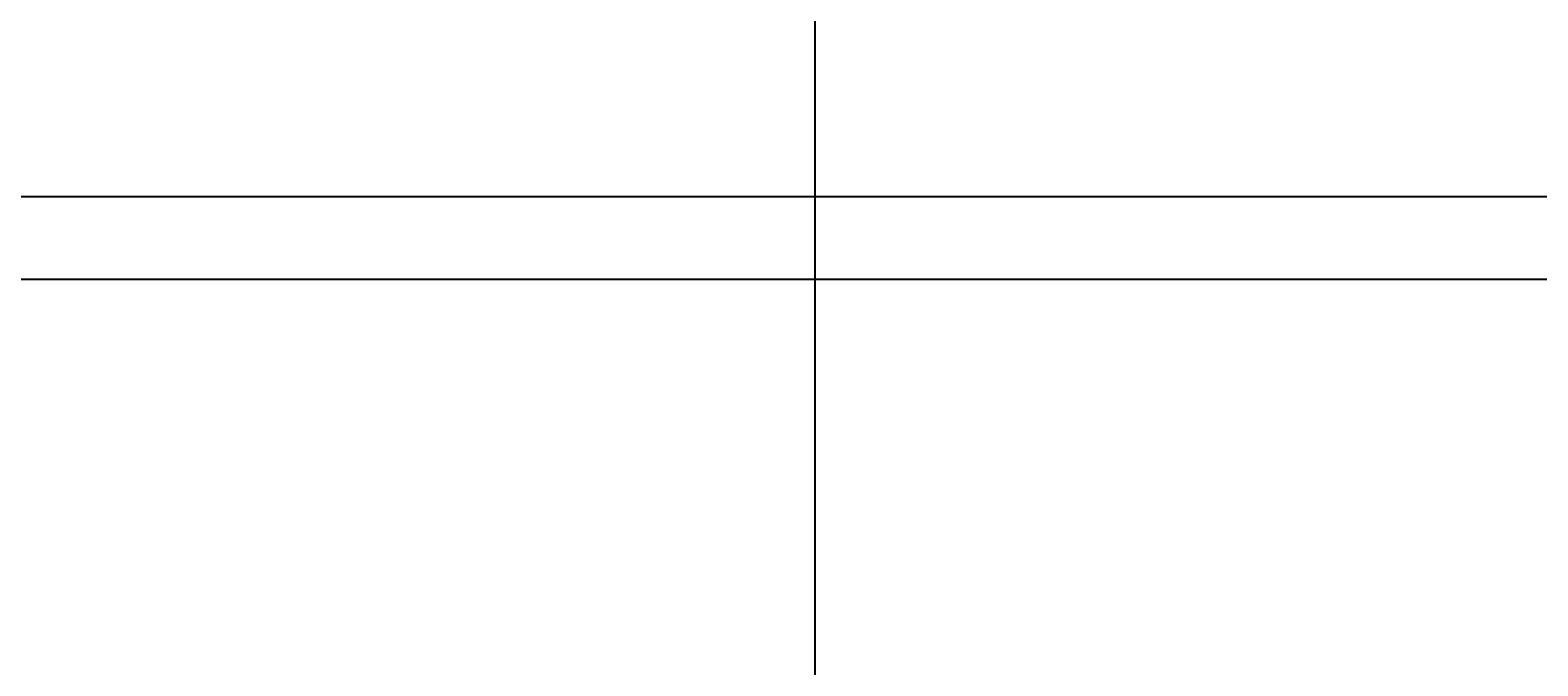
# Model space of a CAD drawing. Units: inches. Extents: x 35362 to 73946, y 43607 to 67532.
# Tile 91 of 134: x 49711 to 50119, y 48793 to 48965. Entities that reach past the tile are written whole.
import ezdxf

# ---------------------------------------------------------------- set-up
doc = ezdxf.new("R2010")
doc.units = ezdxf.units.IN
doc.header["$MEASUREMENT"] = 0
doc.layers.add('A-ANNO-DIMS', color=2, linetype='Continuous', lineweight=18)
doc.styles.get("Standard").update_dxf_attribs({"font": 'arial.ttf'})
doc.dimstyles.get("Standard").update_dxf_attribs({"dimtxt": 0.18, "dimasz": 0.18, "dimexe": 0.18, "dimexo": 0.0625, "dimgap": 0.09, "dimtad": 0, "dimtih": 1, "dimtoh": 1, "dimdec": 4, "dimzin": 0, "dimdsep": 46, "dimtxsty": 'Standard', "dimcen": 0.09, "dimadec": 0, "dimazin": 0, "dimtfac": 1, "dimtdec": 4, "dimtofl": 0, "dimtmove": 0, "dimatfit": 3, "dimfxl": 1, "dimtolj": 1, "dimtzin": 0, "dimarcsym": 0})

# ---------------------------------------------------------------- blocks, each defined once
blk = doc.blocks.new('*D11')
at = {"layer": 'A-ANNO-DIMS', "color": 0, "lineweight": -2, "transparency": 16777216}
for p, q in [((47978.66, 56028.77), (47978.66, 43606.68)), ((53109.76, 56028.77), (53109.76, 43606.68)), ((47978.84, 43606.86), (50543.87, 43606.86)), ((53109.58, 43606.86), (50544.55, 43606.86))]:
    blk.add_line(p, q, dxfattribs=at)
at = {"layer": 'A-ANNO-DIMS', "color": 0, "transparency": 16777216}
for points in [[(47978.84, 43606.89), (47978.84, 43606.83), (47978.66, 43606.86)], [(53109.58, 43606.89), (53109.58, 43606.83), (53109.76, 43606.86)]]:
    blk.add_solid(points, dxfattribs=at)
at = {"layer": 'Defpoints', "color": 0, "transparency": 16777216}
for p in [(47978.66, 56028.84), (53109.76, 56028.84), (53109.76, 43606.86)]:
    blk.add_point(p, dxfattribs=at)
at = {"layer": 'A-ANNO-DIMS', "color": 0, "transparency": 16777216, "insert": (50544.21, 43606.86), "char_height": 0.18, "attachment_point": 5}
blk.add_mtext('\\A1;5131', dxfattribs=at)
blk = doc.blocks.new('*D13')
at = {"layer": 'A-ANNO-DIMS', "color": 0, "lineweight": -2, "transparency": 16777216}
for p, q in [((48373.49, 51694.02), (48373.49, 43606.68)), ((51029.04, 51694.02), (51029.04, 43606.68)), ((48373.67, 43606.86), (49700.8, 43606.86)), ((51028.86, 43606.86), (49701.73, 43606.86))]:
    blk.add_line(p, q, dxfattribs=at)
at = {"layer": 'A-ANNO-DIMS', "color": 0, "transparency": 16777216}
for points in [[(48373.67, 43606.89), (48373.67, 43606.83), (48373.49, 43606.86)], [(51028.86, 43606.89), (51028.86, 43606.83), (51029.04, 43606.86)]]:
    blk.add_solid(points, dxfattribs=at)
at = {"layer": 'Defpoints', "color": 0, "transparency": 16777216}
for p in [(48373.49, 51694.09), (51029.04, 51694.09), (51029.04, 43606.86)]:
    blk.add_point(p, dxfattribs=at)
at = {"layer": 'A-ANNO-DIMS', "color": 0, "transparency": 16777216, "insert": (49701.27, 43606.86), "char_height": 0.18, "attachment_point": 5}
blk.add_mtext('\\A1;2655.6', dxfattribs=at)
blk = doc.blocks.new('*D17')
at = {"layer": 'A-ANNO-DIMS', "color": 0, "lineweight": -2, "transparency": 16777216}
for p, q in [((49923.31, 61293.22), (49923.31, 43606.68)), ((51913.93, 61293.22), (51913.93, 43606.68)), ((49923.49, 43606.86), (50918.16, 43606.86)), ((51913.75, 43606.86), (50919.07, 43606.86))]:
    blk.add_line(p, q, dxfattribs=at)
at = {"layer": 'A-ANNO-DIMS', "color": 0, "transparency": 16777216}
for points in [[(49923.49, 43606.89), (49923.49, 43606.83), (49923.31, 43606.86)], [(51913.75, 43606.89), (51913.75, 43606.83), (51913.93, 43606.86)]]:
    blk.add_solid(points, dxfattribs=at)
at = {"layer": 'Defpoints', "color": 0, "transparency": 16777216}
for p in [(49923.31, 61293.29), (51913.93, 61293.29), (51913.93, 43606.86)]:
    blk.add_point(p, dxfattribs=at)
at = {"layer": 'A-ANNO-DIMS', "color": 0, "transparency": 16777216, "insert": (50918.62, 43606.86), "char_height": 0.18, "attachment_point": 5}
blk.add_mtext('\\A1;1990.6', dxfattribs=at)
blk = doc.blocks.new('*D67')
at = {"layer": 'A-ANNO-DIMS', "color": 0, "lineweight": -2, "transparency": 16777216}
for p, q in [((56873.54, 53351.53), (35361.77, 53351.53)), ((35361.95, 53351.35), (35361.95, 49400.89)), ((35361.95, 45450.07), (35361.95, 49400.53)), ((53793.58, 45449.89), (35361.77, 45449.89))]:
    blk.add_line(p, q, dxfattribs=at)
at = {"layer": 'A-ANNO-DIMS', "color": 0, "transparency": 16777216}
for points in [[(35361.92, 53351.35), (35361.98, 53351.35), (35361.95, 53351.53)], [(35361.92, 45450.07), (35361.98, 45450.07), (35361.95, 45449.89)]]:
    blk.add_solid(points, dxfattribs=at)
at = {"layer": 'Defpoints', "color": 0, "transparency": 16777216}
for p in [(35361.95, 53351.53), (56873.6, 53351.53), (53793.64, 45449.89)]:
    blk.add_point(p, dxfattribs=at)
at = {"layer": 'A-ANNO-DIMS', "color": 0, "transparency": 16777216, "insert": (35361.95, 49400.71), "char_height": 0.18, "attachment_point": 5}
blk.add_mtext('\\A1;7901.6', dxfattribs=at)
blk = doc.blocks.new('*D86')
at = {"layer": 'A-ANNO-DIMS', "color": 0, "lineweight": -2, "transparency": 16777216}
for p, q in [((51285.53, 49320.08), (35361.77, 49320.08)), ((35361.95, 49319.9), (35361.95, 49120.26)), ((35361.95, 48920.26), (35361.95, 49119.9)), ((51285.53, 48920.08), (35361.77, 48920.08))]:
    blk.add_line(p, q, dxfattribs=at)
at = {"layer": 'A-ANNO-DIMS', "color": 0, "transparency": 16777216}
for points in [[(35361.92, 49319.9), (35361.98, 49319.9), (35361.95, 49320.08)], [(35361.92, 48920.26), (35361.98, 48920.26), (35361.95, 48920.08)]]:
    blk.add_solid(points, dxfattribs=at)
at = {"layer": 'Defpoints', "color": 0, "transparency": 16777216}
for p in [(35361.95, 49320.08), (51285.59, 49320.08), (51285.59, 48920.08)]:
    blk.add_point(p, dxfattribs=at)
at = {"layer": 'A-ANNO-DIMS', "color": 0, "transparency": 16777216, "insert": (35361.95, 49120.08), "char_height": 0.18, "attachment_point": 5}
blk.add_mtext('\\A1;400.0', dxfattribs=at)
blk = doc.blocks.new('*D89')
at = {"layer": 'A-ANNO-DIMS', "color": 0, "lineweight": -2, "transparency": 16777216}
for p, q in [((53707.72, 48897.74), (35361.77, 48897.74)), ((35361.95, 48897.56), (35361.95, 48303.16)), ((35361.95, 47708.4), (35361.95, 48302.8)), ((53707.72, 47708.22), (35361.77, 47708.22))]:
    blk.add_line(p, q, dxfattribs=at)
at = {"layer": 'A-ANNO-DIMS', "color": 0, "transparency": 16777216}
for points in [[(35361.92, 48897.56), (35361.98, 48897.56), (35361.95, 48897.74)], [(35361.92, 47708.4), (35361.98, 47708.4), (35361.95, 47708.22)]]:
    blk.add_solid(points, dxfattribs=at)
at = {"layer": 'Defpoints', "color": 0, "transparency": 16777216}
for p in [(53707.78, 48897.74), (35361.95, 47708.22), (53707.78, 47708.22)]:
    blk.add_point(p, dxfattribs=at)
at = {"layer": 'A-ANNO-DIMS', "color": 0, "transparency": 16777216, "insert": (35361.95, 48302.98), "char_height": 0.18, "attachment_point": 5}
blk.add_mtext('\\A1;1189.5', dxfattribs=at)

msp = doc.modelspace()

# ---------------------------------------------------------------- dimensions: what is measured, and where the dimension line sits
at = {"layer": 'A-ANNO-DIMS'}
for base, p1, p2, override, picture, middle in [((51913.931, 43606.859), (49923.307, 61293.286), (51913.931, 61293.286), {"dimdec": 1, "dimlfac": 1, "dimrnd": 0, "dimzin": 0, "dimdsep": 46, "dimlunit": 2}, '*D17', (50918.619, 43606.859)), ((53109.76, 43606.859), (47978.665, 56028.836), (53109.76, 56028.836), {"dimdec": 0, "dimlfac": 1, "dimrnd": 0, "dimzin": 0, "dimdsep": 46, "dimlunit": 2}, '*D11', (50544.212, 43606.859)), ((51029.043, 43606.859), (48373.492, 51694.087), (51029.043, 51694.087), {"dimdec": 1, "dimlfac": 1, "dimrnd": 0, "dimzin": 0, "dimdsep": 46, "dimlunit": 2}, '*D13', (49701.267, 43606.859))]:
    dim = msp.add_linear_dim(base=base, p1=p1, p2=p2, dimstyle='Standard', override=override, dxfattribs=at)
    dim.commit()
    dim.dimension.update_dxf_attribs({"geometry": picture, "text_midpoint": middle})
for base, p1, p2, picture, middle in [((35361.949, 53351.529), (53793.638, 45449.894), (56873.602, 53351.529), '*D67', (35361.949, 49400.712)), ((35361.949, 49320.079), (51285.595, 48920.079), (51285.595, 49320.079), '*D86', (35361.949, 49120.079)), ((35361.949, 47708.216), (53707.781, 48897.738), (53707.781, 47708.216), '*D89', (35361.949, 48302.977))]:
    dim = msp.add_linear_dim(base=base, p1=p1, p2=p2, angle=90, dimstyle='Standard', override={"dimdec": 1, "dimlfac": 1, "dimrnd": 0, "dimzin": 0, "dimdsep": 46, "dimlunit": 2}, dxfattribs=at)
    dim.commit()
    dim.dimension.update_dxf_attribs({"geometry": picture, "text_midpoint": middle})

doc.saveas('drawing.dxf')
